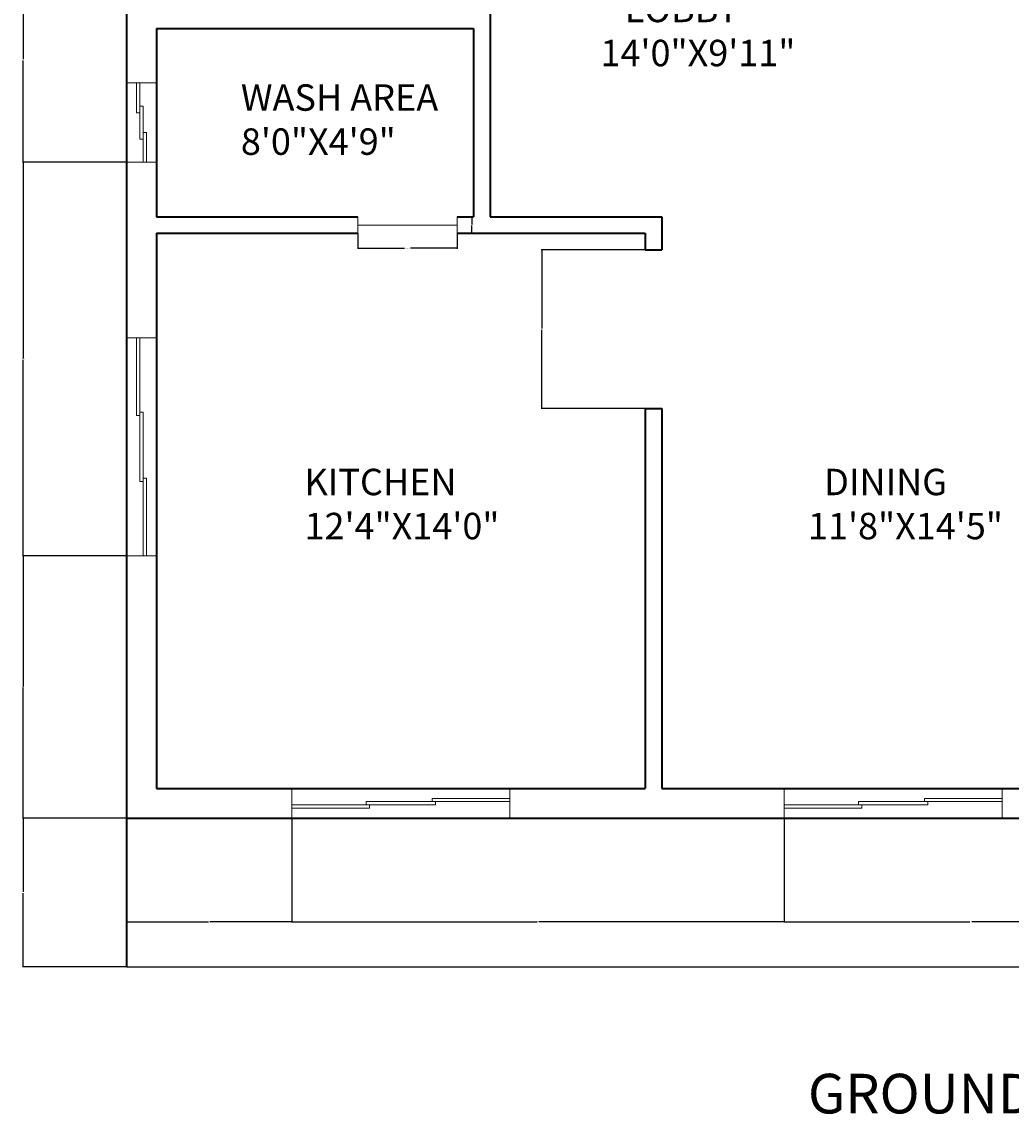
# Model space of a CAD drawing. Units: inches. Extents: x 1569 to 2779, y 1228 to 1844.
# Tile 1 of 6: x 1569 to 1869, y 1228 to 1559. Entities that reach past the tile are written whole.
import ezdxf

# ---------------------------------------------------------------- set-up
doc = ezdxf.new("R2010")
doc.units = ezdxf.units.IN
for name, color, linetype, lineweight in [('A-ANNO-DIMS', 2, 'Continuous', 18), ('A-ANNO-TEXT', 7, 'Continuous', 25), ('A-AREA-IDEN', 7, 'Continuous', 18), ('A-DOOR', 3, 'Continuous', 20), ('A-FLOR-EDGE', 7, 'Continuous', 25), ('A-GLAZ', 5, 'Continuous', 18), ('A-WALL', 7, 'Continuous', 35)]:
    doc.layers.add(name, color=color, linetype=linetype, lineweight=lineweight)
doc.styles.get("Standard").update_dxf_attribs({"font": 'arial.ttf'})
doc.dimstyles.get("Standard").update_dxf_attribs({"dimtxt": 0.18, "dimasz": 0.18, "dimexe": 0.18, "dimexo": 0.0625, "dimgap": 0.09, "dimtad": 0, "dimtih": 1, "dimtoh": 1, "dimdec": 4, "dimzin": 0, "dimdsep": 46, "dimtxsty": 'Standard', "dimcen": 0.09, "dimadec": 0, "dimazin": 0, "dimtfac": 1, "dimtdec": 4, "dimtofl": 0, "dimtmove": 0, "dimatfit": 3, "dimfxl": 1, "dimtolj": 1, "dimtzin": 0, "dimarcsym": 0})

# ---------------------------------------------------------------- blocks, each defined once
blk = doc.blocks.new('WIN-24IN')
for p, q in [((9, 24), (0, 24)), ((3, 24), (3, 15)), ((4, 24), (4, 7)), ((4, 17), (5, 17)), ((5, 17), (5, 0)), ((3, 15), (4, 15)), ((4, 7), (5, 7)), ((5, 9), (6, 9)), ((6, 9), (6, 0)), ((9, 0), (0, 0))]:
    blk.add_line(p, q)
blk = doc.blocks.new('WIN-66IN')
for p, q in [((0, 0), (0, 9)), ((66, 0), (66, 9)), ((0, 4), (43.5, 4)), ((22.5, 5), (66, 5)), ((22.5, 4), (22.5, 5)), ((23.5, 3), (23.5, 4)), ((42.5, 6), (66, 6)), ((42.5, 5), (42.5, 6)), ((43.5, 4), (43.5, 5)), ((0, 3), (23.5, 3))]:
    blk.add_line(p, q)
blk = doc.blocks.new('DOOR-30IN')
for p, q in [((0, 5), (0, 0)), ((30, 5), (30, 0)), ((0, 2.5), (30, 2.5))]:
    blk.add_line(p, q)
blk = doc.blocks.new('*D19')
at = {"layer": 'A-ANNO-DIMS', "color": 0, "lineweight": -2, "transparency": 16777216}
for p, q in [((1671.03, 1494.82), (1671.03, 1490.2)), ((1701.03, 1494.82), (1701.03, 1490.2)), ((1671.21, 1490.38), (1685.1, 1490.38)), ((1700.85, 1490.38), (1686.97, 1490.38))]:
    blk.add_line(p, q, dxfattribs=at)
at = {"layer": 'A-ANNO-DIMS', "color": 0, "transparency": 16777216}
for points in [[(1671.21, 1490.41), (1671.21, 1490.35), (1671.03, 1490.38)], [(1700.85, 1490.41), (1700.85, 1490.35), (1701.03, 1490.38)]]:
    blk.add_solid(points, dxfattribs=at)
at = {"layer": 'Defpoints', "color": 0, "transparency": 16777216}
for p in [(1671.03, 1494.88), (1701.03, 1494.88), (1701.03, 1490.38)]:
    blk.add_point(p, dxfattribs=at)
at = {"layer": 'A-ANNO-DIMS', "color": 0, "transparency": 16777216, "insert": (1686.03, 1490.38), "char_height": 0.18, "attachment_point": 5}
blk.add_mtext('\\A1;DOOR 30 TYP.', dxfattribs=at)
blk = doc.blocks.new('*D20')
at = {"layer": 'A-ANNO-DIMS', "color": 0, "lineweight": -2, "transparency": 16777216}
for p, q in [((1701.09, 1499.88), (1705.71, 1499.88)), ((1705.53, 1499.7), (1705.53, 1497.56)), ((1701.09, 1494.88), (1705.71, 1494.88)), ((1705.53, 1495.06), (1705.53, 1497.2))]:
    blk.add_line(p, q, dxfattribs=at)
at = {"layer": 'A-ANNO-DIMS', "color": 0, "transparency": 16777216}
for points in [[(1705.5, 1499.7), (1705.56, 1499.7), (1705.53, 1499.88)], [(1705.5, 1495.06), (1705.56, 1495.06), (1705.53, 1494.88)]]:
    blk.add_solid(points, dxfattribs=at)
at = {"layer": 'Defpoints', "color": 0, "transparency": 16777216}
for p in [(1701.03, 1499.88), (1705.53, 1499.88), (1701.03, 1494.88)]:
    blk.add_point(p, dxfattribs=at)
at = {"layer": 'A-ANNO-DIMS', "color": 0, "transparency": 16777216, "insert": (1705.53, 1497.38), "char_height": 0.18, "attachment_point": 5}
blk.add_mtext('\\A1;5 TYP.', dxfattribs=at)
blk = doc.blocks.new('*D49')
at = {"layer": 'A-ANNO-DIMS', "color": 0, "lineweight": -2, "transparency": 16777216}
for p, q in [((1600.97, 1317.88), (1569.5, 1317.88)), ((1569.68, 1317.7), (1569.68, 1295.56)), ((1569.68, 1273.06), (1569.68, 1295.2)), ((1600.97, 1272.88), (1569.5, 1272.88))]:
    blk.add_line(p, q, dxfattribs=at)
at = {"layer": 'A-ANNO-DIMS', "color": 0, "transparency": 16777216}
for points in [[(1569.65, 1317.7), (1569.71, 1317.7), (1569.68, 1317.88)], [(1569.65, 1273.06), (1569.71, 1273.06), (1569.68, 1272.88)]]:
    blk.add_solid(points, dxfattribs=at)
at = {"layer": 'Defpoints', "color": 0, "transparency": 16777216}
for p in [(1569.68, 1317.88), (1601.03, 1317.88), (1601.03, 1272.88)]:
    blk.add_point(p, dxfattribs=at)
at = {"layer": 'A-ANNO-DIMS', "color": 0, "transparency": 16777216, "insert": (1569.68, 1295.38), "char_height": 0.18, "attachment_point": 5}
blk.add_mtext('\\A1;45', dxfattribs=at)
blk = doc.blocks.new('*D57')
at = {"layer": 'A-ANNO-DIMS', "color": 0, "lineweight": -2, "transparency": 16777216}
for p, q in [((1601.03, 1317.82), (1601.02, 1286.35)), ((1651.03, 1317.8), (1651.02, 1286.33)), ((1601.2, 1286.53), (1625.8, 1286.52)), ((1650.84, 1286.51), (1626.24, 1286.52))]:
    blk.add_line(p, q, dxfattribs=at)
at = {"layer": 'A-ANNO-DIMS', "color": 0, "transparency": 16777216}
for points in [[(1601.2, 1286.56), (1601.2, 1286.5), (1601.02, 1286.53)], [(1650.84, 1286.54), (1650.84, 1286.48), (1651.02, 1286.51)]]:
    blk.add_solid(points, dxfattribs=at)
at = {"layer": 'Defpoints', "color": 0, "transparency": 16777216}
for p in [(1601.03, 1317.88), (1651.03, 1317.86), (1601.02, 1286.53)]:
    blk.add_point(p, dxfattribs=at)
at = {"layer": 'A-ANNO-DIMS', "color": 0, "transparency": 16777216, "insert": (1626.02, 1286.52), "char_height": 0.18, "attachment_point": 5}
blk.add_mtext('\\A1;50', dxfattribs=at)
blk = doc.blocks.new('*D58')
at = {"layer": 'A-ANNO-DIMS', "color": 0, "lineweight": -2, "transparency": 16777216}
for p, q in [((1651.03, 1317.8), (1651.03, 1286.33)), ((1800.03, 1317.8), (1800.03, 1286.33)), ((1651.21, 1286.51), (1725.25, 1286.51)), ((1799.85, 1286.51), (1725.81, 1286.51))]:
    blk.add_line(p, q, dxfattribs=at)
at = {"layer": 'A-ANNO-DIMS', "color": 0, "transparency": 16777216}
for points in [[(1651.21, 1286.54), (1651.21, 1286.48), (1651.03, 1286.51)], [(1799.85, 1286.54), (1799.85, 1286.48), (1800.03, 1286.51)]]:
    blk.add_solid(points, dxfattribs=at)
at = {"layer": 'Defpoints', "color": 0, "transparency": 16777216}
for p in [(1651.03, 1317.86), (1800.03, 1317.86), (1651.03, 1286.51)]:
    blk.add_point(p, dxfattribs=at)
at = {"layer": 'A-ANNO-DIMS', "color": 0, "transparency": 16777216, "insert": (1725.53, 1286.51), "char_height": 0.18, "attachment_point": 5}
blk.add_mtext('\\A1;149', dxfattribs=at)
blk = doc.blocks.new('*D59')
at = {"layer": 'A-ANNO-DIMS', "color": 0, "lineweight": -2, "transparency": 16777216}
for p, q in [((1800.03, 1317.8), (1800.04, 1286.33)), ((1913.03, 1317.82), (1913.04, 1286.35)), ((1800.22, 1286.51), (1856.26, 1286.52)), ((1912.86, 1286.53), (1856.82, 1286.52))]:
    blk.add_line(p, q, dxfattribs=at)
at = {"layer": 'A-ANNO-DIMS', "color": 0, "transparency": 16777216}
for points in [[(1800.22, 1286.54), (1800.22, 1286.48), (1800.04, 1286.51)], [(1912.86, 1286.56), (1912.86, 1286.5), (1913.04, 1286.53)]]:
    blk.add_solid(points, dxfattribs=at)
at = {"layer": 'Defpoints', "color": 0, "transparency": 16777216}
for p in [(1800.03, 1317.86), (1913.03, 1317.88), (1800.04, 1286.51)]:
    blk.add_point(p, dxfattribs=at)
at = {"layer": 'A-ANNO-DIMS', "color": 0, "transparency": 16777216, "insert": (1856.54, 1286.52), "char_height": 0.18, "attachment_point": 5}
blk.add_mtext('\\A1;113', dxfattribs=at)
blk = doc.blocks.new('*D61')
at = {"layer": 'A-ANNO-DIMS', "color": 0, "lineweight": -2, "transparency": 16777216}
for p, q in [((1600.97, 1397.25), (1569.5, 1397.25)), ((1569.68, 1397.07), (1569.68, 1357.75)), ((1569.68, 1318.06), (1569.68, 1357.38)), ((1600.97, 1317.88), (1569.5, 1317.88))]:
    blk.add_line(p, q, dxfattribs=at)
at = {"layer": 'A-ANNO-DIMS', "color": 0, "transparency": 16777216}
for points in [[(1569.65, 1397.07), (1569.71, 1397.07), (1569.68, 1397.25)], [(1569.65, 1318.06), (1569.71, 1318.06), (1569.68, 1317.88)]]:
    blk.add_solid(points, dxfattribs=at)
at = {"layer": 'Defpoints', "color": 0, "transparency": 16777216}
for p in [(1569.68, 1397.25), (1601.03, 1397.25), (1601.03, 1317.88)]:
    blk.add_point(p, dxfattribs=at)
at = {"layer": 'A-ANNO-DIMS', "color": 0, "transparency": 16777216, "insert": (1569.68, 1357.56), "char_height": 0.18, "attachment_point": 5}
blk.add_mtext('\\A1;79.37', dxfattribs=at)
blk = doc.blocks.new('*D62')
at = {"layer": 'A-ANNO-DIMS', "color": 0, "lineweight": -2, "transparency": 16777216}
for p, q in [((1600.97, 1516.38), (1569.5, 1516.38)), ((1569.68, 1516.2), (1569.68, 1457)), ((1569.68, 1397.43), (1569.68, 1456.63)), ((1600.97, 1397.25), (1569.5, 1397.25))]:
    blk.add_line(p, q, dxfattribs=at)
at = {"layer": 'A-ANNO-DIMS', "color": 0, "transparency": 16777216}
for points in [[(1569.65, 1516.2), (1569.71, 1516.2), (1569.68, 1516.38)], [(1569.65, 1397.43), (1569.71, 1397.43), (1569.68, 1397.25)]]:
    blk.add_solid(points, dxfattribs=at)
at = {"layer": 'Defpoints', "color": 0, "transparency": 16777216}
for p in [(1569.68, 1516.38), (1601.03, 1516.38), (1601.03, 1397.25)]:
    blk.add_point(p, dxfattribs=at)
at = {"layer": 'A-ANNO-DIMS', "color": 0, "transparency": 16777216, "insert": (1569.68, 1456.81), "char_height": 0.18, "attachment_point": 5}
blk.add_mtext('\\A1;119.13', dxfattribs=at)
blk = doc.blocks.new('*D63')
at = {"layer": 'A-ANNO-DIMS', "color": 0, "lineweight": -2, "transparency": 16777216}
for p, q in [((1600.97, 1578.38), (1569.5, 1578.38)), ((1569.68, 1578.2), (1569.68, 1547.56)), ((1569.68, 1516.56), (1569.68, 1547.2)), ((1600.97, 1516.38), (1569.5, 1516.38))]:
    blk.add_line(p, q, dxfattribs=at)
at = {"layer": 'A-ANNO-DIMS', "color": 0, "transparency": 16777216}
for points in [[(1569.65, 1578.2), (1569.71, 1578.2), (1569.68, 1578.38)], [(1569.65, 1516.56), (1569.71, 1516.56), (1569.68, 1516.38)]]:
    blk.add_solid(points, dxfattribs=at)
at = {"layer": 'Defpoints', "color": 0, "transparency": 16777216}
for p in [(1569.68, 1578.38), (1601.03, 1578.38), (1601.03, 1516.38)]:
    blk.add_point(p, dxfattribs=at)
at = {"layer": 'A-ANNO-DIMS', "color": 0, "transparency": 16777216, "insert": (1569.68, 1547.38), "char_height": 0.18, "attachment_point": 5}
blk.add_mtext('\\A1;62', dxfattribs=at)
blk = doc.blocks.new('*D81')
at = {"layer": 'A-ANNO-DIMS', "color": 0, "lineweight": -2, "transparency": 16777216}
for p, q in [((1757.97, 1489.88), (1726.5, 1489.88)), ((1726.68, 1489.7), (1726.68, 1466.06)), ((1726.68, 1442.06), (1726.68, 1465.7)), ((1757.97, 1441.88), (1726.5, 1441.88))]:
    blk.add_line(p, q, dxfattribs=at)
at = {"layer": 'A-ANNO-DIMS', "color": 0, "transparency": 16777216}
for points in [[(1726.65, 1489.7), (1726.71, 1489.7), (1726.68, 1489.88)], [(1726.65, 1442.06), (1726.71, 1442.06), (1726.68, 1441.88)]]:
    blk.add_solid(points, dxfattribs=at)
at = {"layer": 'Defpoints', "color": 0, "transparency": 16777216}
for p in [(1726.68, 1489.88), (1758.03, 1489.88), (1758.03, 1441.88)]:
    blk.add_point(p, dxfattribs=at)
at = {"layer": 'A-ANNO-DIMS', "color": 0, "transparency": 16777216, "insert": (1726.68, 1465.88), "char_height": 0.18, "attachment_point": 5}
blk.add_mtext('\\A1;48', dxfattribs=at)

msp = doc.modelspace()

# ---------------------------------------------------------------- linework, layer by layer
at = {"layer": 'A-FLOR-EDGE'}
msp.add_line((1601.032, 1272.8785), (2141.032, 1272.8785), dxfattribs=at)
at = {"layer": 'A-WALL'}
for p, q in [((1601.032, 1812.8785), (1601.032, 1272.8785)), ((1711.032, 1566.8785), (1711.032, 1499.8785)), ((1610.032, 1556.8785), (1706.032, 1556.8785)), ((1610.032, 1556.8785), (1610.032, 1499.8785)), ((1706.032, 1556.8785), (1706.032, 1499.8785)), ((1610.032, 1499.8785), (1671.032, 1499.8785)), ((1701.032, 1499.8785), (1706.032, 1499.8785)), ((1711.032, 1499.8785), (1763.032, 1499.8785)), ((1763.032, 1499.8785), (1763.032, 1489.8785)), ((1610.032, 1494.8785), (1671.032, 1494.8785)), ((1610.032, 1494.8785), (1610.032, 1326.8785)), ((1701.032, 1494.8785), (1758.032, 1494.8785)), ((1758.032, 1494.8785), (1758.032, 1489.8785)), ((1758.032, 1489.8785), (1763.032, 1489.8785)), ((1758.032, 1441.8785), (1763.032, 1441.8785)), ((1758.032, 1441.8785), (1758.032, 1326.8785)), ((1763.032, 1441.8785), (1763.032, 1326.8785)), ((1610.032, 1326.8785), (1758.032, 1326.8785)), ((1763.032, 1326.8785), (1903.032, 1326.8785)), ((1601.032, 1317.8785), (1913.032, 1317.8785))]:
    msp.add_line(p, q, dxfattribs=at)

# ---------------------------------------------------------------- block references
at = {"layer": 'A-DOOR'}
msp.add_blockref('DOOR-30IN', (1671.032, 1494.8785), dxfattribs=at)
at = {"layer": 'A-GLAZ'}
for name, p in [('WIN-24IN', (1601.032, 1516.3785)), ('WIN-66IN', (1651.032, 1317.863)), ('WIN-66IN', (1800.032, 1317.863))]:
    msp.add_blockref(name, p, dxfattribs=at)
at = {"layer": 'A-GLAZ', "rotation": 269.999999999999}
msp.add_blockref('WIN-66IN', (1601.032, 1463.2502), dxfattribs=at)

# ---------------------------------------------------------------- texts
at = {"layer": 'A-ANNO-TEXT', "insert": (1807.2679, 1240.4981), "char_height": 12, "attachment_point": 1}
msp.add_mtext_dynamic_manual_height_columns('GROUND FLOOR PLAN', width=187.856256, gutter_width=12.5, heights=[0], dxfattribs=at)
at = {"layer": 'A-AREA-IDEN', "char_height": 8, "attachment_point": 1}
for s, width, heights, insert in [('   LOBBY\\P14\'0"X9\'11"', 101.861325, [21.6444], (1744.451, 1566.78)), ('WASH AREA\\P8\'0"X4\'9"', 82.13469, [0], (1635.6037, 1539.9634)), ('KITCHEN\\P12\'4"X14\'0"', 101.861325, [0], (1654.8676, 1423.6131)), ('  DINING\\P11\'8"X14\'5"', 101.861325, [0], (1807.2679, 1423.6131))]:
    msp.add_mtext_dynamic_manual_height_columns(s, width=width, gutter_width=12.5, heights=heights, dxfattribs=dict(at, insert=insert))

# ---------------------------------------------------------------- dimensions: what is measured, and where the dimension line sits
at = {"layer": 'A-ANNO-DIMS'}
for base, p1, p2, angle, override, picture, middle in [((1569.682, 1578.3785), (1601.032, 1516.3785), (1601.032, 1578.3785), 90, {"dimdec": 0, "dimlfac": 1, "dimrnd": 0, "dimzin": 0, "dimdsep": 46, "dimlunit": 2}, '*D63', (1569.682, 1547.3785)), ((1569.682, 1516.3785), (1601.032, 1397.2502), (1601.032, 1516.3785), 90, {"dimdec": 2, "dimlfac": 1, "dimrnd": 0, "dimzin": 0, "dimdsep": 46, "dimlunit": 2}, '*D62', (1569.682, 1456.8143)), ((1726.682, 1489.8785), (1758.032, 1441.8785), (1758.032, 1489.8785), 90, {"dimdec": 0, "dimlfac": 1, "dimrnd": 0, "dimzin": 0, "dimdsep": 46, "dimlunit": 2}, '*D81', (1726.682, 1465.8785)), ((1569.682, 1397.2502), (1601.032, 1317.8785), (1601.032, 1397.2502), 90, {"dimdec": 2, "dimlfac": 1, "dimrnd": 0, "dimzin": 0, "dimdsep": 46, "dimlunit": 2}, '*D61', (1569.682, 1357.5643)), ((1569.682, 1317.8785), (1601.032, 1272.8785), (1601.032, 1317.8785), 90, {"dimdec": 0, "dimlfac": 1, "dimrnd": 0, "dimzin": 0, "dimdsep": 46, "dimlunit": 2}, '*D49', (1569.682, 1295.3785)), ((1601.0223, 1286.5285), (1651.032, 1317.863), (1601.032, 1317.8785), 179.98229, {"dimdec": 0, "dimlfac": 1, "dimrnd": 0, "dimzin": 0, "dimdsep": 46, "dimlunit": 2}, '*D57', (1626.0223, 1286.5208)), ((1651.032, 1286.513), (1800.032, 1317.863), (1651.032, 1317.863), 180, {"dimdec": 0, "dimlfac": 1, "dimrnd": 0, "dimzin": 0, "dimdsep": 46, "dimlunit": 2}, '*D58', (1725.532, 1286.513)), ((1800.0363, 1286.513), (1913.032, 1317.8785), (1800.032, 1317.863), 180.007836, {"dimdec": 0, "dimlfac": 1, "dimrnd": 0, "dimzin": 0, "dimdsep": 46, "dimlunit": 2}, '*D59', (1856.5363, 1286.5208))]:
    dim = msp.add_linear_dim(base=base, p1=p1, p2=p2, angle=angle, dimstyle='Standard', override=override, dxfattribs=at)
    dim.commit()
    dim.dimension.update_dxf_attribs({"geometry": picture, "text_midpoint": middle})
dim = msp.add_linear_dim(base=(1705.532, 1499.8785), p1=(1701.032, 1494.8785), p2=(1701.032, 1499.8785), angle=90, text='<> TYP.', dimstyle='Standard', override={"dimdec": 0, "dimlfac": 1, "dimrnd": 0, "dimzin": 0, "dimdsep": 46, "dimlunit": 2}, dxfattribs=at)
dim.commit()
dim.dimension.update_dxf_attribs({"geometry": '*D20', "text_midpoint": (1705.532, 1497.3785)})
dim = msp.add_linear_dim(base=(1701.032, 1490.3785), p1=(1671.032, 1494.8785), p2=(1701.032, 1494.8785), text='DOOR <> TYP.', dimstyle='Standard', override={"dimdec": 0, "dimlfac": 1, "dimrnd": 0, "dimzin": 0, "dimdsep": 46, "dimlunit": 2}, dxfattribs=at)
dim.commit()
dim.dimension.update_dxf_attribs({"geometry": '*D19', "text_midpoint": (1686.032, 1490.3785)})

doc.saveas('drawing.dxf')
